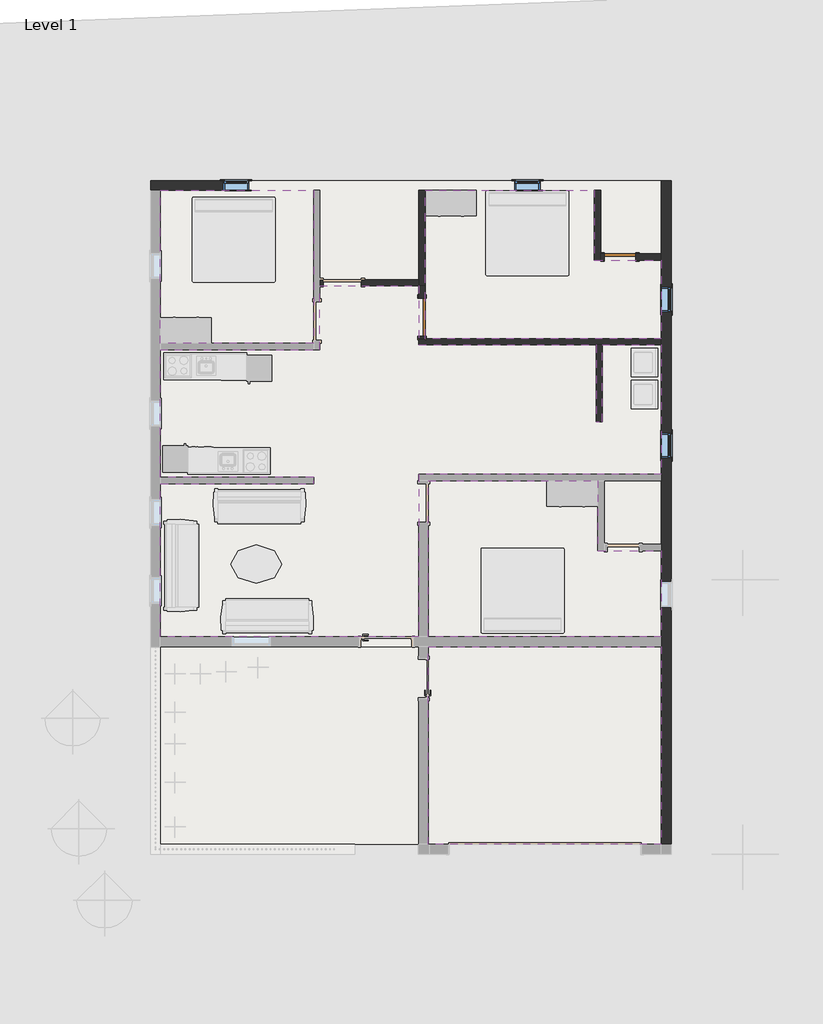
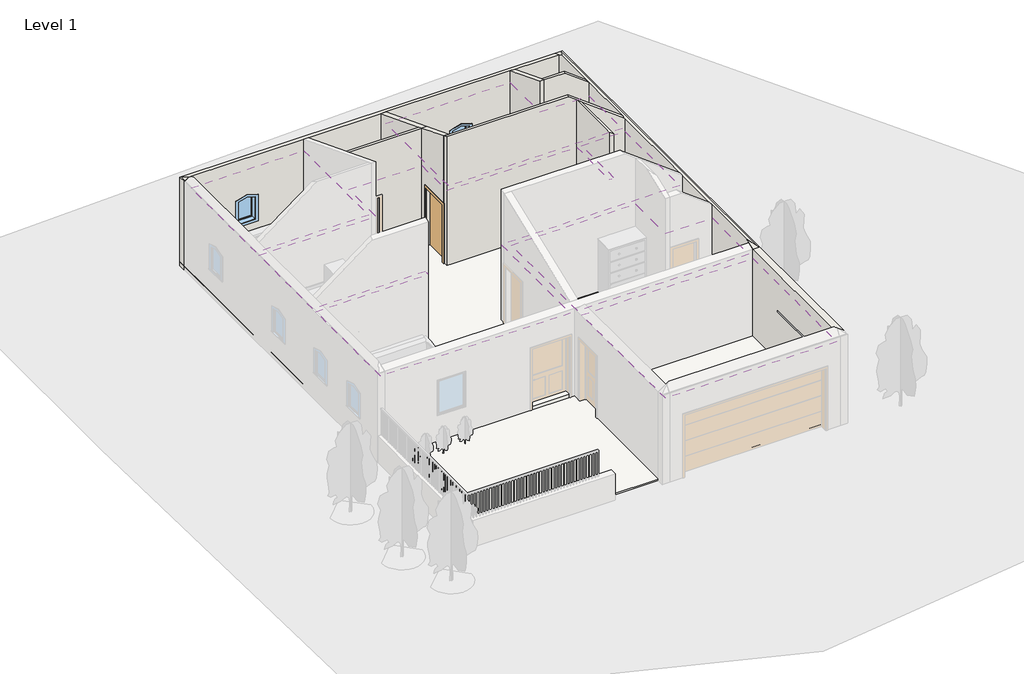
# One storey, part 2 of 3: 9 walls, 5 coverings, 4 windows, 3 slabs, 2 doors.
"""IFC4 building model written with IfcOpenShell, lengths in millimetres."""

from ifc_helpers import new_model, si_unit, frame, origin, origin_with_axes, place, context, project, spatial, polyline, circle_curve, outline, extrude, faceted_brep, transform, mapped, element, save
from ifc_brep_helpers import plane_surface, revolved_surface, advanced_brep
from components import single_flush_25_e2b13fe9, door_16372e1c, window_fb83c811

model = new_model("IFC4")

# Units and contexts
model_context = context("Model", 3, world=origin())
ifc_project = project(units=[si_unit("LENGTHUNIT", "METRE", prefix="MILLI")], contexts=[model_context])

# Site, building, storey
site = spatial("IfcSite", under=ifc_project)
building = spatial("IfcBuilding", under=site)
storey = spatial("IfcBuildingStorey", under=building, Name="Level 1", Elevation=0.0)

# Coverings
placement = place(None, origin())
element("IfcCovering", 1, ObjectType="2' x 4' ACT System", at=placement, inside=storey, context=model_context, shape_type="SweptSolid", body=[
    extrude(outline(polyline([(-2236.1368615, 5136.6670221), (-826.4368615, 5136.6670221), (-826.4368615, 2050.5670221), (-6617.6368615, 2050.5670221), (-6617.6368615, -1835.6329779), (-12789.8368615, -1835.6329779), (-12789.8368615, 1821.9670221), (-9132.2368615, 1821.9670221), (-9132.2368615, 1974.3670221), (-12789.8368615, 1974.3670221), (-12789.8368615, 5022.3670221), (-8979.8368615, 5022.3670221), (-8979.8368615, 6546.3670221), (-6617.6368615, 6546.3670221), (-6617.6368615, 5136.6670221), (-2388.5368615, 5136.6670221), (-2388.5368615, 3307.8670221), (-2236.1368615, 3307.8670221), (-2236.1368615, 5136.6670221)])), frame((0.0, 0.0, 2743.2), z_axis=(0.0, 0.0, 1.0), x_axis=(1.0, 0.0, 0.0)), (0.0, 0.0, 1.0), 57.15),
])
element("IfcCovering", 2, ObjectType="2' x 4' ACT System", at=placement, inside=storey, context=model_context, shape_type="SweptSolid", body=[
    extrude(outline(polyline([(-12789.8368615, 8832.3670221), (-9132.2368615, 8832.3670221), (-9132.2368615, 5174.7670221), (-12789.8368615, 5174.7670221), (-12789.8368615, 8832.3670221)])), frame((0.0, 0.0, 2743.2), z_axis=(0.0, 0.0, 1.0), x_axis=(1.0, 0.0, 0.0)), (0.0, 0.0, 1.0), 57.15),
])
element("IfcCovering", 3, ObjectType="2' x 4' ACT System", at=placement, inside=storey, context=model_context, shape_type="SweptSolid", body=[
    extrude(outline(polyline([(-6465.2368615, 6622.5670221), (-6465.2368615, 8832.3670221), (-2426.6368615, 8832.3670221), (-2426.6368615, 7155.9670221), (-826.4368615, 7155.9670221), (-826.4368615, 5289.0670221), (-6465.2368615, 5289.0670221), (-6465.2368615, 6622.5670221)])), frame((0.0, 0.0, 2743.2), z_axis=(0.0, 0.0, 1.0), x_axis=(1.0, 0.0, 0.0)), (0.0, 0.0, 1.0), 57.15),
])
element("IfcCovering", 4, ObjectType="2' x 4' ACT System", at=placement, inside=storey, context=model_context, shape_type="SweptSolid", body=[
    extrude(outline(polyline([(-826.4368615, 221.7670221), (-826.4368615, -1835.6329779), (-6389.0368615, -1835.6329779), (-6389.0368615, 1898.1670221), (-2350.4368615, 1898.1670221), (-2350.4368615, 221.7670221), (-826.4368615, 221.7670221)])), frame((0.0, 0.0, 2743.2), z_axis=(0.0, 0.0, 1.0), x_axis=(1.0, 0.0, 0.0)), (0.0, 0.0, 1.0), 57.15),
])
element("IfcCovering", 5, ObjectType="2' x 4' ACT System", at=placement, inside=storey, context=model_context, shape_type="SweptSolid", body=[
    extrude(outline(polyline([(-826.4368615, -2064.2329779), (-826.4368615, -6788.6329779), (-6389.0368615, -6788.6329779), (-6389.0368615, -2064.2329779), (-826.4368615, -2064.2329779)])), frame((0.0, 0.0, 2743.2), z_axis=(0.0, 0.0, 1.0), x_axis=(1.0, 0.0, 0.0)), (0.0, 0.0, 1.0), 57.15),
])

# Doors
single_flush_25_shape = single_flush_25_e2b13fe9(model_context)
element("IfcDoor", 6, ObjectType="Single-Flush : 25'", at=placement, inside=storey, context=model_context, shape_type="MappedRepresentation", body=[
    mapped(single_flush_25_shape, transform((-1817.0368615, 7232.1670221, 0.0), x_axis=(-1.0, 0.0, 0.0), y_axis=(0.0, -1.0, 0.0), z_axis=(0.0, 0.0, 1.0))),
])
door_shape = door_16372e1c(model_context)
element("IfcDoor", 7, ObjectType="Single-Flush : 36\" x 84\"", at=placement, inside=storey, context=model_context, shape_type="MappedRepresentation", body=[
    mapped(door_shape, transform((-6541.4368615, 5797.0670221, 0.0), x_axis=(0.0, -1.0, 0.0), y_axis=(1.0, 0.0, 0.0), z_axis=(0.0, 0.0, 1.0))),
])

# Slabs
element("IfcSlab", 8, ObjectType="3\"", at=placement, inside=storey, context=model_context, shape_type="SweptSolid", body=[
    extrude(outline(polyline([(-6401.7368615, -2076.9329779), (-6401.7368615, -6788.6329779), (-12789.8368615, -6788.6329779), (-12789.8368615, -2076.9329779), (-6401.7368615, -2076.9329779)])), frame((0.0, 0.0, -25.4), z_axis=(0.0, 0.0, 1.0), x_axis=(1.0, 0.0, 0.0)), (0.0, 0.0, 1.0), 76.2),
])
element("IfcSlab", 9, ObjectType="3\"", at=placement, inside=storey, context=model_context, shape_type="SweptSolid", body=[
    extrude(outline(polyline([(-826.4368615, -2064.2329779), (-826.4368615, -6788.6329779), (-6389.0368615, -6788.6329779), (-6389.0368615, -2064.2329779), (-826.4368615, -2064.2329779)])), origin_with_axes(), (0.0, 0.0, 1.0), 76.2),
])
element("IfcSlab", 10, ObjectType="6\"", at=placement, inside=storey, context=model_context, shape_type="SweptSolid", body=[
    extrude(outline(polyline([(-597.8368615, 9060.9670221), (-597.8368615, -2064.2329779), (-13018.4368615, -2064.2329779), (-13018.4368615, 9060.9670221), (-597.8368615, 9060.9670221)])), origin_with_axes(), (0.0, 0.0, 1.0), 152.4),
])

# Walls
element("IfcWall", 11, ObjectType="6\"", at=placement, inside=storey, context=model_context, shape_type="Brep", body=[
    faceted_brep([(-6617.6368615, 8832.3670221, 0.0), (-6617.6368615, 6698.7670221, 0.0), (-6617.6368615, 6546.3670221, 0.0), (-6617.6368615, 6546.3670221, 4025.0611069), (-6617.6368615, 6698.7670221, 3965.8452822), (-6617.6368615, 8832.3670221, 3136.823737), (-6465.2368615, 8832.3670221, 0.0), (-6465.2368615, 8832.3670221, 3136.823737), (-6465.2368615, 6546.3670221, 4025.0611069), (-6465.2368615, 6546.3670221, 0.0)], [[[0, 1, 2, 3, 4, 5]], [[6, 7, 8, 9]], [[2, 1, 0, 6, 9]], [[0, 5, 7, 6]], [[3, 2, 9, 8]], [[5, 4, 3, 8, 7]]]),
])
element("IfcWall", 12, ObjectType="6\"", at=placement, inside=storey, context=model_context, shape_type="Brep", body=[
    faceted_brep([(-8903.6368615, 6698.7670221, 2133.6), (-8903.6368615, 6698.7670221, 0.0), (-8979.8368615, 6698.7670221, 0.0), (-8979.8368615, 6698.7670221, 3965.8452822), (-6617.6368615, 6698.7670221, 3965.8452822), (-6617.6368615, 6698.7670221, 0.0), (-7989.2368615, 6698.7670221, 0.0), (-7989.2368615, 6698.7670221, 2133.6), (-8979.8368615, 6546.3670221, 0.0), (-8903.6368615, 6546.3670221, 0.0), (-8903.6368615, 6546.3670221, 2133.6), (-7989.2368615, 6546.3670221, 2133.6), (-7989.2368615, 6546.3670221, 0.0), (-6617.6368615, 6546.3670221, 0.0), (-6617.6368615, 6546.3670221, 4025.0611069), (-8979.8368615, 6546.3670221, 4025.0611069)], [[[0, 1, 2, 3, 4, 5, 6, 7]], [[8, 9, 10, 11, 12, 13, 14, 15]], [[6, 5, 13, 12]], [[2, 1, 9, 8]], [[5, 4, 14, 13]], [[3, 2, 8, 15]], [[10, 9, 1, 0]], [[11, 10, 0, 7]], [[12, 11, 7, 6]], [[4, 3, 15, 14]]]),
])
element("IfcWall", 13, ObjectType="6\"", at=placement, inside=storey, context=model_context, shape_type="Brep", body=[
    faceted_brep([(-826.4368615, 5289.0670221, 0.0), (-6465.2368615, 5289.0670221, 0.0), (-6617.6368615, 5289.0670221, 0.0), (-6617.6368615, 5289.0670221, 4513.5916603), (-6465.2368615, 5289.0670221, 4513.5916603), (-2587.9589779, 5289.0670221, 4513.5916603), (-826.4368615, 5289.0670221, 3192.4500731), (-826.4368615, 5136.6670221, 0.0), (-826.4368615, 5136.6670221, 3192.4500731), (-2236.1368615, 5136.6670221, 4249.7250731), (-2388.5368615, 5136.6670221, 4364.0250731), (-2666.9134107, 5136.6670221, 4572.807485), (-6617.6368615, 5136.6670221, 4572.807485), (-6617.6368615, 5136.6670221, 0.0), (-2388.5368615, 5136.6670221, 0.0), (-2236.1368615, 5136.6670221, 0.0)], [[[0, 1, 2, 3, 4, 5, 6]], [[7, 8, 9, 10, 11, 12, 13, 14, 15]], [[2, 1, 0, 7, 15, 14, 13]], [[0, 6, 8, 7]], [[3, 2, 13, 12]], [[6, 5, 11, 10, 9, 8]], [[5, 4, 3, 12, 11]]]),
])
element("IfcWall", 14, ObjectType="6\"", at=placement, inside=storey, context=model_context, shape_type="SweptSolid", body=[
    extrude(outline(polyline([(5339.8670221, 2133.6), (5339.8670221, 0.0), (5289.0670221, 0.0), (5289.0670221, 4513.5916603), (6546.3670221, 4025.0611069), (6546.3670221, 0.0), (6254.2670221, 0.0), (6254.2670221, 2133.6), (5339.8670221, 2133.6)])), frame((-6617.6368615, 0.0, 0.0), z_axis=(1.0, 0.0, 0.0), x_axis=(0.0, 1.0, 0.0)), (0.0, 0.0, 1.0), 152.4),
])
element("IfcWall", 15, ObjectType="6\"", at=placement, inside=storey, context=model_context, shape_type="Brep", body=[
    faceted_brep([(-2426.6368615, 8832.3670221, 0.0), (-2426.6368615, 7155.9670221, 0.0), (-2426.6368615, 7155.9670221, 3788.1978082), (-2426.6368615, 8832.3670221, 3136.823737), (-2274.2368615, 8832.3670221, 0.0), (-2274.2368615, 8832.3670221, 3136.823737), (-2274.2368615, 7308.3670221, 3728.9819836), (-2274.2368615, 7155.9670221, 3788.1978082), (-2274.2368615, 7155.9670221, 0.0), (-2274.2368615, 7308.3670221, 0.0)], [[[0, 1, 2, 3]], [[4, 5, 6, 7, 8, 9]], [[1, 0, 4, 9, 8]], [[0, 3, 5, 4]], [[2, 1, 8, 7]], [[3, 2, 7, 6, 5]]]),
])
element("IfcWall", 16, ObjectType="6\"", at=placement, inside=storey, context=model_context, shape_type="Brep", body=[
    faceted_brep([(-2274.2368615, 7155.9670221, 0.0), (-2198.0368615, 7155.9670221, 0.0), (-2198.0368615, 7155.9670221, 2133.6), (-1436.0368615, 7155.9670221, 2133.6), (-1436.0368615, 7155.9670221, 0.0), (-826.4368615, 7155.9670221, 0.0), (-826.4368615, 7155.9670221, 3192.4500731), (-1620.7671751, 7155.9670221, 3788.1978082), (-2274.2368615, 7155.9670221, 3788.1978082), (-2198.0368615, 7308.3670221, 2133.6), (-2198.0368615, 7308.3670221, 0.0), (-2274.2368615, 7308.3670221, 0.0), (-2274.2368615, 7308.3670221, 3728.9819836), (-1541.8127422, 7308.3670221, 3728.9819836), (-826.4368615, 7308.3670221, 3192.4500731), (-826.4368615, 7308.3670221, 0.0), (-1436.0368615, 7308.3670221, 0.0), (-1436.0368615, 7308.3670221, 2133.6)], [[[0, 1, 2, 3, 4, 5, 6, 7, 8]], [[9, 10, 11, 12, 13, 14, 15, 16, 17]], [[16, 15, 5, 4]], [[11, 10, 1, 0]], [[0, 8, 12, 11]], [[6, 5, 15, 14]], [[2, 1, 10, 9]], [[3, 2, 9, 17]], [[4, 3, 17, 16]], [[8, 7, 13, 12]], [[7, 6, 14, 13]]]),
])
element("IfcWall", 17, ObjectType="6\"", at=placement, inside=storey, context=model_context, shape_type="SweptSolid", body=[
    extrude(outline(polyline([(4364.0250731, -2388.5368615), (0.0, -2388.5368615), (0.0, -2236.1368615), (4249.7250731, -2236.1368615), (4364.0250731, -2388.5368615)])), frame((0.0, 3307.8670221, 0.0), z_axis=(0.0, 1.0, 0.0), x_axis=(0.0, 0.0, 1.0)), (0.0, 0.0, 1.0), 1828.8),
])
element("IfcWall", 18, ObjectType="9\"", at=placement, inside=storey, context=model_context, shape_type="AdvancedBrep", body=[
    advanced_brep(
    [(-13018.4368615, 8832.3670221, 0.0), (-12789.8368615, 8832.3670221, 0.0), (-9132.2368615, 8832.3670221, 0.0), (-8979.8368615, 8832.3670221, 0.0), (-6617.6368615, 8832.3670221, 0.0), (-6465.2368615, 8832.3670221, 0.0), (-2426.6368615, 8832.3670221, 0.0), (-2274.2368615, 8832.3670221, 0.0), (-826.4368615, 8832.3670221, 0.0), (-826.4368615, 8832.3670221, 3136.823737), (-2274.2368615, 8832.3670221, 3136.823737), (-2426.6368615, 8832.3670221, 3136.823737), (-6465.2368615, 8832.3670221, 3136.823737), (-6617.6368615, 8832.3670221, 3136.823737), (-8979.8368615, 8832.3670221, 3136.823737), (-9132.2368615, 8832.3670221, 3136.823737), (-12789.8368615, 8832.3670221, 3136.823737), (-12864.0053096, 8832.3670221, 3136.823737), (-12982.4369589, 8832.3670221, 3048.0), (-13018.4368615, 8832.3670221, 3048.0), (-10675.2868615, 8832.3670221, 1747.1290861), (-10675.2868615, 8832.3670221, 914.4), (-11284.8868615, 8832.3670221, 914.4), (-11284.8868615, 8832.3670221, 1747.1290861), (-10980.0868615, 8832.3670221, 1828.8), (-3722.0368615, 8832.3670221, 1747.1290861), (-3722.0368615, 8832.3670221, 914.4), (-4331.6368615, 8832.3670221, 914.4), (-4331.6368615, 8832.3670221, 1747.1290861), (-4026.8368615, 8832.3670221, 1828.8), (-13018.4368615, 9060.9670221, 0.0), (-13018.4368615, 9060.9670221, 3048.0), (-12982.4369589, 9060.9670221, 3048.0), (-826.4368615, 9060.9670221, 3048.0), (-826.4368615, 9060.9670221, 0.0), (-10675.2868615, 9060.9670221, 1747.1290861), (-10980.0868615, 9060.9670221, 1828.8), (-11284.8868615, 9060.9670221, 1747.1290861), (-11284.8868615, 9060.9670221, 914.4), (-10675.2868615, 9060.9670221, 914.4), (-3722.0368615, 9060.9670221, 1747.1290861), (-4026.8368615, 9060.9670221, 1828.8), (-4331.6368615, 9060.9670221, 1747.1290861), (-4331.6368615, 9060.9670221, 914.4), (-3722.0368615, 9060.9670221, 914.4)],
    [
        (0, 1),
        (1, 2),
        (2, 3),
        (3, 4),
        (4, 5),
        (5, 6),
        (6, 7),
        (7, 8),
        (8, 9),
        (9, 10),
        (10, 11),
        (11, 12),
        (12, 13),
        (13, 14),
        (14, 15),
        (15, 16),
        (16, 17),
        (17, 18),
        (18, 19),
        (19, 0),
        (20, 21),
        (21, 22),
        (22, 23),
        (23, 24, circle_curve(frame((-10980.0868615, 8832.3670221, 1219.2), z_axis=(0.0, 1.0, 0.0), x_axis=(1.0, 0.0, 0.0)), 609.6)),
        (24, 20, circle_curve(frame((-10980.0868615, 8832.3670221, 1219.2), z_axis=(0.0, 1.0, 0.0), x_axis=(1.0, 0.0, 0.0)), 609.6)),
        (25, 26),
        (26, 27),
        (27, 28),
        (28, 29, circle_curve(frame((-4026.8368615, 8832.3670221, 1219.2), z_axis=(0.0, 1.0, 0.0), x_axis=(1.0, 0.0, 0.0)), 609.6)),
        (29, 25, circle_curve(frame((-4026.8368615, 8832.3670221, 1219.2), z_axis=(0.0, 1.0, 0.0), x_axis=(1.0, 0.0, 0.0)), 609.6)),
        (30, 31),
        (31, 32),
        (32, 33),
        (33, 34),
        (34, 30),
        (35, 36, circle_curve(frame((-10980.0868615, 9060.9670221, 1219.2), z_axis=(0.0, -1.0, 0.0), x_axis=(1.0, 0.0, 0.0)), 609.6)),
        (36, 37, circle_curve(frame((-10980.0868615, 9060.9670221, 1219.2), z_axis=(0.0, -1.0, 0.0), x_axis=(1.0, 0.0, 0.0)), 609.6)),
        (37, 38),
        (38, 39),
        (39, 35),
        (40, 41, circle_curve(frame((-4026.8368615, 9060.9670221, 1219.2), z_axis=(0.0, -1.0, 0.0), x_axis=(1.0, 0.0, 0.0)), 609.6)),
        (41, 42, circle_curve(frame((-4026.8368615, 9060.9670221, 1219.2), z_axis=(0.0, -1.0, 0.0), x_axis=(1.0, 0.0, 0.0)), 609.6)),
        (42, 43),
        (43, 44),
        (44, 40),
        (0, 30),
        (34, 8),
        (19, 31),
        (33, 9),
        (32, 17),
        (18, 32),
        (20, 35),
        (39, 21),
        (38, 22),
        (37, 23),
        (36, 24),
        (25, 40),
        (44, 26),
        (43, 27),
        (42, 28),
        (41, 29),
    ],
    [
        plane_surface(frame((-15342.5368615, 8832.3670221, 0.0), z_axis=(0.0, -1.0, 0.0), x_axis=(1.0, 0.0, 0.0))),
        plane_surface(frame((-15342.5368615, 9060.9670221, 0.0), z_axis=(0.0, 1.0, 0.0), x_axis=(-1.0, 0.0, 0.0))),
        plane_surface(frame((-12904.1368615, 8832.3670221, 0.0), z_axis=(0.0, 0.0, -1.0), x_axis=(0.0, 1.0, 0.0))),
        plane_surface(frame((-13018.4368615, 11385.0670221, 0.0), z_axis=(-1.0, 0.0, 0.0), x_axis=(0.0, -1.0, 0.0))),
        plane_surface(frame((-826.4368615, 8946.6670221, 0.0), z_axis=(1.0, 0.0, 0.0), x_axis=(0.0, -1.0, 0.0))),
        plane_surface(frame((-633.8367641, 9060.9670221, 3048.0), z_axis=(0.0, 0.3621761357767564, 0.932109675238819), x_axis=(-1.0, 0.0, 0.0))),
        plane_surface(frame((-597.8368615, 9060.9670221, 3048.0), z_axis=(0.0, 0.0, 1.0), x_axis=(-1.0, 0.0, 0.0))),
        plane_surface(frame((-12982.4369589, 9060.9670221, 3048.0), z_axis=(-0.6000000000000011, 0.0, 0.7999999999999992), x_axis=(0.0, -1.0, 0.0))),
        plane_surface(frame((-10675.2868615, 8832.3670221, 1747.1290861), z_axis=(-1.0, 0.0, 0.0), x_axis=(0.0, 1.0, 0.0))),
        plane_surface(frame((-10675.2868615, 8832.3670221, 914.4), z_axis=(0.0, 0.0, 1.0), x_axis=(0.0, 1.0, 0.0))),
        plane_surface(frame((-11284.8868615, 8832.3670221, 914.4), z_axis=(1.0, 0.0, 0.0), x_axis=(0.0, 1.0, 0.0))),
        revolved_surface(polyline([(-10370.4868615, 9060.9670221, 1219.2), (-10370.4868615, 8832.3670221, 1219.2)]), (-10980.0868615, 8832.3670221, 1219.2), (0.0, 1.0, 0.0)),
        plane_surface(frame((-3722.0368615, 8832.3670221, 1747.1290861), z_axis=(-1.0, 0.0, 0.0), x_axis=(0.0, 1.0, 0.0))),
        plane_surface(frame((-3722.0368615, 8832.3670221, 914.4), z_axis=(0.0, 0.0, 1.0), x_axis=(0.0, 1.0, 0.0))),
        plane_surface(frame((-4331.6368615, 8832.3670221, 914.4), z_axis=(1.0, 0.0, 0.0), x_axis=(0.0, 1.0, 0.0))),
        revolved_surface(polyline([(-3417.2368615, 9060.9670221, 1219.2), (-3417.2368615, 8832.3670221, 1219.2)]), (-4026.8368615, 8832.3670221, 1219.2), (0.0, 1.0, 0.0)),
    ],
    [
        (0, [[1, 2, 3, 4, 5, 6, 7, 8, 9, 10, 11, 12, 13, 14, 15, 16, 17, 18, 19, 20], [21, 22, 23, 24, 25], [26, 27, 28, 29, 30]]),
        (1, [[31, 32, 33, 34, 35], [36, 37, 38, 39, 40], [41, 42, 43, 44, 45]]),
        (2, [[-8, -7, -6, -5, -4, -3, -2, -1, 46, -35, 47]]),
        (3, [[-20, 48, -31, -46]]),
        (4, [[-9, -47, -34, 49]]),
        (5, [[-17, -16, -15, -14, -13, -12, -11, -10, -49, -33, 50]]),
        (6, [[-19, 51, -32, -48]]),
        (7, [[-18, -50, -51]]),
        (8, [[-21, 52, -40, 53]]),
        (9, [[-22, -53, -39, 54]]),
        (10, [[-23, -54, -38, 55]]),
        (11, [[-24, -55, -37, 56]]),
        (11, [[-25, -56, -36, -52]]),
        (12, [[-26, 57, -45, 58]]),
        (13, [[-27, -58, -44, 59]]),
        (14, [[-28, -59, -43, 60]]),
        (15, [[-29, -60, -42, 61]]),
        (15, [[-30, -61, -41, -57]]),
    ],
),
])
element("IfcWall", 19, ObjectType="9\"", at=placement, inside=storey, context=model_context, shape_type="AdvancedBrep", body=[
    advanced_brep(
    [(-826.4368615, 9060.9670221, 0.0), (-826.4368615, 8832.3670221, 0.0), (-826.4368615, 7308.3670221, 0.0), (-826.4368615, 7155.9670221, 0.0), (-826.4368615, 5289.0670221, 0.0), (-826.4368615, 5136.6670221, 0.0), (-826.4368615, 2050.5670221, 0.0), (-826.4368615, 1898.1670221, 0.0), (-826.4368615, 374.1670221, 0.0), (-826.4368615, 221.7670221, 0.0), (-826.4368615, -1835.6329779, 0.0), (-826.4368615, -2064.2329779, 0.0), (-826.4368615, -6788.6329779, 0.0), (-826.4368615, -6788.6329779, 3048.0), (-826.4368615, -2064.2329779, 3048.0), (-826.4368615, -1835.6329779, 3136.823737), (-826.4368615, -1692.4710163, 3192.4500731), (-826.4368615, 221.7670221, 3192.4500731), (-826.4368615, 374.1670221, 3192.4500731), (-826.4368615, 1898.1670221, 3192.4500731), (-826.4368615, 2050.5670221, 3192.4500731), (-826.4368615, 5136.6670221, 3192.4500731), (-826.4368615, 5289.0670221, 3192.4500731), (-826.4368615, 7155.9670221, 3192.4500731), (-826.4368615, 7308.3670221, 3192.4500731), (-826.4368615, 8689.2050605, 3192.4500731), (-826.4368615, 8832.3670221, 3136.823737), (-826.4368615, 9060.9670221, 3048.0), (-826.4368615, 5917.7170221, 1747.1290861), (-826.4368615, 5917.7170221, 914.4), (-826.4368615, 6527.3170221, 914.4), (-826.4368615, 6527.3170221, 1747.1290861), (-826.4368615, 6222.5170221, 1828.8), (-826.4368615, 2431.5670221, 1747.1290861), (-826.4368615, 2431.5670221, 914.4), (-826.4368615, 3041.1670221, 914.4), (-826.4368615, 3041.1670221, 1747.1290861), (-826.4368615, 2736.3670221, 1828.8), (-826.4368615, -1130.7829779, 1747.1290861), (-826.4368615, -1130.7829779, 914.4), (-826.4368615, -521.1829779, 914.4), (-826.4368615, -521.1829779, 1747.1290861), (-826.4368615, -825.9829779, 1828.8), (-597.8368615, 9060.9670221, 0.0), (-597.8368615, 9060.9670221, 3048.0), (-597.8368615, -2064.2329779, 3048.0), (-597.8368615, -6788.6329779, 3048.0), (-597.8368615, -6788.6329779, 0.0), (-597.8368615, 5917.7170221, 1747.1290861), (-597.8368615, 6222.5170221, 1828.8), (-597.8368615, 6527.3170221, 1747.1290861), (-597.8368615, 6527.3170221, 914.4), (-597.8368615, 5917.7170221, 914.4), (-597.8368615, 2431.5670221, 1747.1290861), (-597.8368615, 2736.3670221, 1828.8), (-597.8368615, 3041.1670221, 1747.1290861), (-597.8368615, 3041.1670221, 914.4), (-597.8368615, 2431.5670221, 914.4), (-597.8368615, -1130.7829779, 1747.1290861), (-597.8368615, -825.9829779, 1828.8), (-597.8368615, -521.1829779, 1747.1290861), (-597.8368615, -521.1829779, 914.4), (-597.8368615, -1130.7829779, 914.4), (-633.8367641, 9060.9670221, 3048.0), (-633.8367641, -2064.2329779, 3048.0)],
    [
        (0, 1),
        (1, 2),
        (2, 3),
        (3, 4),
        (4, 5),
        (5, 6),
        (6, 7),
        (7, 8),
        (8, 9),
        (9, 10),
        (10, 11),
        (11, 12),
        (12, 13),
        (13, 14),
        (14, 15),
        (15, 16),
        (16, 17),
        (17, 18),
        (18, 19),
        (19, 20),
        (20, 21),
        (21, 22),
        (22, 23),
        (23, 24),
        (24, 25),
        (25, 26),
        (26, 27),
        (27, 0),
        (28, 29),
        (29, 30),
        (30, 31),
        (31, 32, circle_curve(frame((-826.4368615, 6222.5170221, 1219.2), z_axis=(1.0, 0.0, 0.0), x_axis=(0.0, -1.0, 0.0)), 609.6)),
        (32, 28, circle_curve(frame((-826.4368615, 6222.5170221, 1219.2), z_axis=(1.0, 0.0, 0.0), x_axis=(0.0, -1.0, 0.0)), 609.6)),
        (33, 34),
        (34, 35),
        (35, 36),
        (36, 37, circle_curve(frame((-826.4368615, 2736.3670221, 1219.2), z_axis=(1.0, 0.0, 0.0), x_axis=(0.0, -1.0, 0.0)), 609.6)),
        (37, 33, circle_curve(frame((-826.4368615, 2736.3670221, 1219.2), z_axis=(1.0, 0.0, 0.0), x_axis=(0.0, -1.0, 0.0)), 609.6)),
        (38, 39),
        (39, 40),
        (40, 41),
        (41, 42, circle_curve(frame((-826.4368615, -825.9829779, 1219.2), z_axis=(1.0, 0.0, 0.0), x_axis=(0.0, -1.0, 0.0)), 609.6)),
        (42, 38, circle_curve(frame((-826.4368615, -825.9829779, 1219.2), z_axis=(1.0, 0.0, 0.0), x_axis=(0.0, -1.0, 0.0)), 609.6)),
        (43, 44),
        (44, 45),
        (45, 46),
        (46, 47),
        (47, 43),
        (48, 49, circle_curve(frame((-597.8368615, 6222.5170221, 1219.2), z_axis=(-1.0, 0.0, 0.0), x_axis=(0.0, -1.0, 0.0)), 609.6)),
        (49, 50, circle_curve(frame((-597.8368615, 6222.5170221, 1219.2), z_axis=(-1.0, 0.0, 0.0), x_axis=(0.0, -1.0, 0.0)), 609.6)),
        (50, 51),
        (51, 52),
        (52, 48),
        (53, 54, circle_curve(frame((-597.8368615, 2736.3670221, 1219.2), z_axis=(-1.0, 0.0, 0.0), x_axis=(0.0, -1.0, 0.0)), 609.6)),
        (54, 55, circle_curve(frame((-597.8368615, 2736.3670221, 1219.2), z_axis=(-1.0, 0.0, 0.0), x_axis=(0.0, -1.0, 0.0)), 609.6)),
        (55, 56),
        (56, 57),
        (57, 53),
        (58, 59, circle_curve(frame((-597.8368615, -825.9829779, 1219.2), z_axis=(-1.0, 0.0, 0.0), x_axis=(0.0, -1.0, 0.0)), 609.6)),
        (59, 60, circle_curve(frame((-597.8368615, -825.9829779, 1219.2), z_axis=(-1.0, 0.0, 0.0), x_axis=(0.0, -1.0, 0.0)), 609.6)),
        (60, 61),
        (61, 62),
        (62, 58),
        (0, 43),
        (47, 12),
        (27, 63),
        (63, 44),
        (46, 13),
        (45, 64),
        (64, 14),
        (25, 63),
        (16, 64),
        (64, 63),
        (28, 48),
        (52, 29),
        (51, 30),
        (50, 31),
        (49, 32),
        (33, 53),
        (57, 34),
        (56, 35),
        (55, 36),
        (54, 37),
        (38, 58),
        (62, 39),
        (61, 40),
        (60, 41),
        (59, 42),
    ],
    [
        plane_surface(frame((-826.4368615, 8946.6670221, 0.0), z_axis=(-1.0, 0.0, 0.0), x_axis=(0.0, -1.0, 0.0))),
        plane_surface(frame((-597.8368615, 8946.6670221, 0.0), z_axis=(1.0, 0.0, 0.0), x_axis=(0.0, 1.0, 0.0))),
        plane_surface(frame((-826.4368615, 8946.6670221, 0.0), z_axis=(0.0, 0.0, -1.0), x_axis=(1.0, 0.0, 0.0))),
        plane_surface(frame((-15342.5368615, 9060.9670221, 0.0), z_axis=(0.0, 1.0, 0.0), x_axis=(-1.0, 0.0, 0.0))),
        plane_surface(frame((1726.2631385, -6788.6329779, 0.0), z_axis=(0.0, -1.0, 0.0), x_axis=(-1.0, 0.0, 0.0))),
        plane_surface(frame((-826.4368615, -6902.9329779, 3048.0), z_axis=(0.0, 0.0, 1.0), x_axis=(1.0, 0.0, 0.0))),
        plane_surface(frame((-633.8367641, 9060.9670221, 3048.0), z_axis=(0.0, 0.3621761357767564, 0.932109675238819), x_axis=(-1.0, 0.0, 0.0))),
        plane_surface(frame((-633.8367641, -2064.2329779, 3048.0), z_axis=(0.5999999999999996, 0.0, 0.8000000000000003), x_axis=(0.0, 1.0, 0.0))),
        plane_surface(frame((-12982.4369589, -2064.2329779, 3048.0), z_axis=(0.0, -0.3621761357767551, 0.9321096752388195), x_axis=(1.0, 0.0, 0.0))),
        plane_surface(frame((-597.8368615, 9060.9670221, 3048.0), z_axis=(0.0, 0.0, 1.0), x_axis=(-1.0, 0.0, 0.0))),
        plane_surface(frame((-826.4368615, 5917.7170221, 1747.1290861), z_axis=(0.0, 1.0, 0.0), x_axis=(1.0, 0.0, 0.0))),
        plane_surface(frame((-826.4368615, 5917.7170221, 914.4), z_axis=(0.0, 0.0, 1.0), x_axis=(1.0, 0.0, 0.0))),
        plane_surface(frame((-826.4368615, 6527.3170221, 914.4), z_axis=(0.0, -1.0, 0.0), x_axis=(1.0, 0.0, 0.0))),
        revolved_surface(polyline([(-597.8368615, 5612.9170220999995, 1219.2), (-826.4368615, 5612.9170220999995, 1219.2)]), (-826.4368615, 6222.5170221, 1219.2), (1.0, 0.0, 0.0)),
        plane_surface(frame((-826.4368615, 2431.5670221, 1747.1290861), z_axis=(0.0, 1.0, 0.0), x_axis=(1.0, 0.0, 0.0))),
        plane_surface(frame((-826.4368615, 2431.5670221, 914.4), z_axis=(0.0, 0.0, 1.0), x_axis=(1.0, 0.0, 0.0))),
        plane_surface(frame((-826.4368615, 3041.1670221, 914.4), z_axis=(0.0, -1.0, 0.0), x_axis=(1.0, 0.0, 0.0))),
        revolved_surface(polyline([(-597.8368615, 2126.7670221000003, 1219.2), (-826.4368615, 2126.7670221000003, 1219.2)]), (-826.4368615, 2736.3670221, 1219.2), (1.0, 0.0, 0.0)),
        plane_surface(frame((-826.4368615, -1130.7829779, 1747.1290861), z_axis=(0.0, 1.0, 0.0), x_axis=(1.0, 0.0, 0.0))),
        plane_surface(frame((-826.4368615, -1130.7829779, 914.4), z_axis=(0.0, 0.0, 1.0), x_axis=(1.0, 0.0, 0.0))),
        plane_surface(frame((-826.4368615, -521.1829779, 914.4), z_axis=(0.0, -1.0, 0.0), x_axis=(1.0, 0.0, 0.0))),
        revolved_surface(polyline([(-597.8368615, -1435.5829779, 1219.2), (-826.4368615, -1435.5829779, 1219.2)]), (-826.4368615, -825.9829779, 1219.2), (1.0, 0.0, 0.0)),
    ],
    [
        (0, [[1, 2, 3, 4, 5, 6, 7, 8, 9, 10, 11, 12, 13, 14, 15, 16, 17, 18, 19, 20, 21, 22, 23, 24, 25, 26, 27, 28], [29, 30, 31, 32, 33], [34, 35, 36, 37, 38], [39, 40, 41, 42, 43]]),
        (1, [[44, 45, 46, 47, 48], [49, 50, 51, 52, 53], [54, 55, 56, 57, 58], [59, 60, 61, 62, 63]]),
        (2, [[-12, -11, -10, -9, -8, -7, -6, -5, -4, -3, -2, -1, 64, -48, 65]]),
        (3, [[-28, 66, 67, -44, -64]]),
        (4, [[-13, -65, -47, 68]]),
        (5, [[-14, -68, -46, 69, 70]]),
        (6, [[-27, -26, 71, -66]]),
        (7, [[-25, -24, -23, -22, -21, -20, -19, -18, -17, 72, 73, -71]]),
        (8, [[-16, -15, -70, -72]]),
        (9, [[-69, -45, -67, -73]]),
        (10, [[-29, 74, -53, 75]]),
        (11, [[-30, -75, -52, 76]]),
        (12, [[-31, -76, -51, 77]]),
        (13, [[-32, -77, -50, 78]]),
        (13, [[-33, -78, -49, -74]]),
        (14, [[-34, 79, -58, 80]]),
        (15, [[-35, -80, -57, 81]]),
        (16, [[-36, -81, -56, 82]]),
        (17, [[-37, -82, -55, 83]]),
        (17, [[-38, -83, -54, -79]]),
        (18, [[-39, 84, -63, 85]]),
        (19, [[-40, -85, -62, 86]]),
        (20, [[-41, -86, -61, 87]]),
        (21, [[-42, -87, -60, 88]]),
        (21, [[-43, -88, -59, -84]]),
    ],
),
])

# Windows
window_shape = window_fb83c811(model_context)
element("IfcWindow", 20, ObjectType="Archtop with Trim : 24\" x 36\"", at=placement, inside=storey, context=model_context, shape_type="MappedRepresentation", body=[
    mapped(window_shape, transform((-10992.0671595, 8946.6670221, 0.0), x_axis=(1.0, 0.0, 0.0), y_axis=(0.0, 1.0, 0.0), z_axis=(0.0, 0.0, 1.0))),
])
element("IfcWindow", 21, ObjectType="Archtop with Trim : 24\" x 36\"", at=placement, inside=storey, context=model_context, shape_type="MappedRepresentation", body=[
    mapped(window_shape, transform((-4038.8171595, 8946.6670221, 0.0), x_axis=(1.0, 0.0, 0.0), y_axis=(0.0, 1.0, 0.0), z_axis=(0.0, 0.0, 1.0))),
])
element("IfcWindow", 22, ObjectType="Archtop with Trim : 24\" x 36\"", at=placement, inside=storey, context=model_context, shape_type="MappedRepresentation", body=[
    mapped(window_shape, transform((-712.1368615, 6234.4973201, 0.0), x_axis=(0.0, -1.0, 0.0), y_axis=(1.0, 0.0, 0.0), z_axis=(0.0, 0.0, 1.0))),
])
element("IfcWindow", 23, ObjectType="Archtop with Trim : 24\" x 36\"", at=placement, inside=storey, context=model_context, shape_type="MappedRepresentation", body=[
    mapped(window_shape, transform((-712.1368615, 2748.3473201, 0.0), x_axis=(0.0, -1.0, 0.0), y_axis=(1.0, 0.0, 0.0), z_axis=(0.0, 0.0, 1.0))),
])

save(model, "model.ifc")

# Revit data of these elements
# Type "2' x 4' ACT System"
#   Assembly Code = "C3030210"
#   built-in parameter 1002203 = 1 (stored number, unit not read)
#   built-in parameter 1002202 = 1 (stored number, unit not read)
#   Layers, outside or top first: 0' - 1 5/8" "Default" (function 1); 0' - 0 5/8" "Acoustic Ceiling Tile 24 x 48" (function 5)
# Type "Single-Flush : 25'"
#   Type Mark = "8"
#   Construction Type Id = "MDOOR"
#   Assembly Code = "C1020"
#   Analytic Construction = "Metal"
#   Thickness = 0' - 2"
#   Heat Transfer Coefficient (U) = 0.651978 BTU/(h·ft²·°F)
#   Height = 7' - 0"
#   Trim Projection Ext = 0' - 1"
#   Trim Projection Int = 0' - 1"
#   Trim Width = 0' - 3"
#   Width = 2' - 6"
#   Define Thermal Properties by = 1
#   Door Material = Door - Panel
#   Frame Material = Door - Frame
#   Visual Light Transmittance = 0
#   Solar Heat Gain Coefficient = 0
#   Function = (empty or 0)
#   Wall Closure = (empty or 0)
# Type "Single-Flush : 36\" x 84\""
#   Type Mark = "1"
#   Construction Type Id = "MDOOR"
#   Assembly Code = "C1020"
#   Analytic Construction = "Metal"
#   Thickness = 0' - 2"
#   Heat Transfer Coefficient (U) = 0.651978 BTU/(h·ft²·°F)
#   Height = 7' - 0"
#   Trim Projection Ext = 0' - 1"
#   Trim Projection Int = 0' - 1"
#   Trim Width = 0' - 3"
#   Width = 3' - 0"
#   Define Thermal Properties by = 1
#   Door Material = Door - Panel
#   Frame Material = Door - Frame
#   Visual Light Transmittance = 0
#   Solar Heat Gain Coefficient = 0
#   Function = (empty or 0)
#   Wall Closure = (empty or 0)
# Type "3\""
#   Assembly Code = "B1010"
#   Function = 0
#   Layers, outside or top first: 0' - 3" "GRASS" (function 1)
# Type "6\""
#   Assembly Code = "B1010"
#   Function = 0
#   Layers, outside or top first: 0' - 6" "FLOOR" (function 1)
# Type "6\""
#   Assembly Code = "B2010"
#   Layers, outside or top first: 0' - 6" "INT WALL" (function 1)
# Type "9\""
#   Assembly Code = "B2010"
#   Layers, outside or top first: 0' - 9" "EXT WALL" (function 1)
# Type "Archtop with Trim : 24\" x 36\""
#   Type Mark = "10"
#   Construction Type Id = "GSP4R"
#   Assembly Code = "B2020100"
#   Analytic Construction = "1/8 in Pilkington single glazing"
#   Visual Light Transmittance = 0.9
#   Solar Heat Gain Coefficient = 0.78
#   Heat Transfer Coefficient (U) = 0.6496 BTU/(h·ft²·°F)
#   Height = 3' - 0"
#   Radius = 2' - 0"
#   Default Sill Height = 3' - 0"
#   Trim Projection - Ext. = 0' - 0 1/2"
#   Trim Projection - Int. = 0' - 0 3/4"
#   Trim Width - Exterior = 0' - 3 1/2"
#   Trim Width - Interior = 0' - 3 1/2"
#   Width = 2' - 0"
#   Define Thermal Properties by = 1
#   Glass Pane Material = Glass
#   Sash Material = Sash
#   Trim Exterior Material = Trim
#   Trim Interior Material = Trim
#   Wall Closure = (empty or 0)
# Elements 1, 2, 3, 4, 5 (IfcCovering, "2' x 4' ACT System")
#   Height Offset From Level = 9' - 0"
#   Phase Created = New Construction
#   Materials on its faces: "Acoustic Ceiling Tile 24 x 48", "Default"
# Element 6 (IfcDoor, "Single-Flush : 25'")
#   Phase Created = New Construction
#   Materials on its faces: "Door - Frame", "Door - Panel"
# Element 7 (IfcDoor, "Single-Flush : 36\" x 84\"")
#   Phase Created = New Construction
#   Materials on its faces: "Door - Frame", "Door - Panel"
# Element 8 (IfcSlab, "3\"")
#   Height Offset From Level = 0' - 2"
#   Phase Created = New Construction
#   Materials on its faces: "GRASS"
# Element 9 (IfcSlab, "3\"")
#   Height Offset From Level = 0' - 3"
#   Phase Created = New Construction
#   Materials on its faces: "GRASS"
# Element 10 (IfcSlab, "6\"")
#   Height Offset From Level = 0' - 6"
#   Phase Created = New Construction
#   Materials on its faces: "FLOOR"
# Elements 11, 12, 13, 14, 15, 16, 17 (IfcWall, "6\"")
#   Top Offset = 0' - 0"
#   Base Offset = 0' - 0"
#   Unconnected Height = 10' - 0"
#   wall height = 10' - 0"
#   Phase Created = New Construction
#   Base Constraint = Level 1
#   Materials on its faces: "INT WALL"
# Elements 18, 19 (IfcWall, "9\"")
#   Top Offset = 0' - 0"
#   Base Offset = 0' - 0"
#   Unconnected Height = 10' - 0"
#   wall height = 10' - 0"
#   Phase Created = New Construction
#   Base Constraint = Level 1
#   Materials on its faces: "EXT WALL"
# Element 20 (IfcWindow, "Archtop with Trim : 24\" x 36\"")
#   Mark = "6"
#   Phase Created = New Construction
#   Materials on its faces: "Sash", "Trim", "Glass"
# Element 21 (IfcWindow, "Archtop with Trim : 24\" x 36\"")
#   Mark = "7"
#   Phase Created = New Construction
#   Materials on its faces: "Sash", "Trim", "Glass"
# Element 22 (IfcWindow, "Archtop with Trim : 24\" x 36\"")
#   Mark = "8"
#   Phase Created = New Construction
#   Materials on its faces: "Sash", "Trim", "Glass"
# Element 23 (IfcWindow, "Archtop with Trim : 24\" x 36\"")
#   Mark = "9"
#   Phase Created = New Construction
#   Materials on its faces: "Sash", "Trim", "Glass"
# Materials
#   "Default": colour RGB 127 127 127, transparency 0
#   "Acoustic Ceiling Tile 24 x 48": class "Generic", colour RGB 229 229 229, transparency 0, Description = "Acoustic Ceiling Tile 24 x 48", Cost = 0
#   "Door - Panel": class "Wood", colour RGB 210 159 95, transparency 0
#   "Door - Frame": colour RGB 118 70 51, transparency 0
#   "GRASS": class "Generic", colour RGB 127 136 91, transparency 0, Cost = 0
#   "FLOOR": class "Generic", colour RGB 141 116 85, transparency 0, Cost = 0
#   "INT WALL": class "Generic", colour RGB 175 172 159, transparency 0, Cost = 0
#   "EXT WALL": class "Generic", colour RGB 216 216 204, transparency 0, Cost = 0
#   "Glass": class "Glass", colour RGB 0 128 192, transparency 0.75, Description = "Soda Lime Glass", Cost = 0
#   "Sash": class "Wood", colour RGB 224 178 126, transparency 0
#   "Trim": class "Wood", colour RGB 224 178 126, transparency 0
